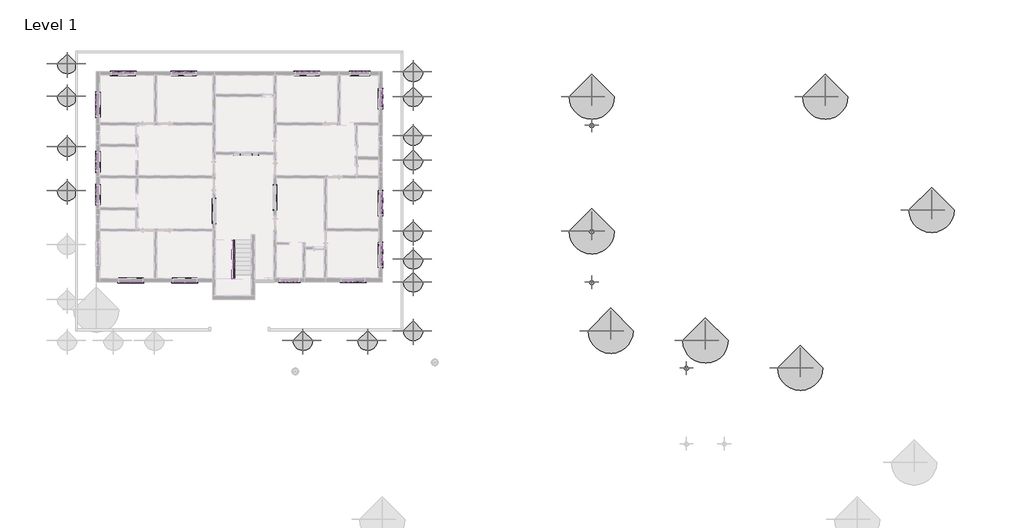
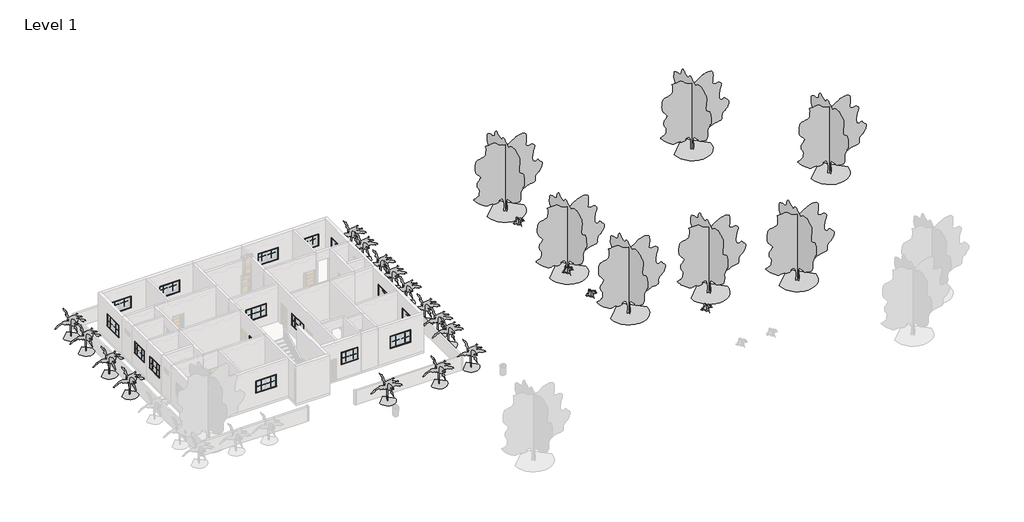
# One storey, part 5 of 5: 68 proxies, 26 geographic elements, 3 members.
"""IFC4 building model written with IfcOpenShell, lengths in millimetres."""

from ifc_helpers import new_model, si_unit, frame, origin, place, context, project, spatial, polyline, outline, extrude, transform, mapped, element, save
from components import m_muntin_pattern_2x2_m_muntin_pattern_2x2_9352d081, m_muntin_pattern_2x2_m_muntin_pattern_2x2_5c2cbe28, m_muntin_pattern_2x2_m_muntin_pattern_2x2_2357e71d, m_muntin_pattern_2x2_m_muntin_pattern_2x2_302d8f29, m_trim_window_exterior_flat_with_sill_e3533f3c, m_trim_window_exterior_flat_with_sill_6ae8fed8, m_trim_window_interior_flat_picture_frame_7d8195fd, m_trim_window_interior_flat_picture_frame_fffd0b6f, m_rpc_plant_tropical_agave_0_45_meters_eb57889b, m_rpc_tree_tropical_australian_tree_fern_1_8_meters_0203a3dd, rpc_tree_deciduous_american_beech_20_b3c041c8

model = new_model("IFC4")

# Units and contexts
model_context = context("Model", 3, world=origin())
ifc_project = project(units=[si_unit("LENGTHUNIT", "METRE", prefix="MILLI")], contexts=[model_context])

# Site, building, storey
site = spatial("IfcSite", under=ifc_project)
building = spatial("IfcBuilding", under=site)
storey = spatial("IfcBuildingStorey", under=building, Name="Level 1", Elevation=0.0)

# Proxies
placement = place(None, origin())
m_muntin_pattern_2x2_m_muntin_pattern_2x2_shape = m_muntin_pattern_2x2_m_muntin_pattern_2x2_9352d081(model_context)
element("IfcBuildingElementProxy", 1, Name="M_Muntin Pattern_2x2 : M_Muntin Pattern_2x2", ObjectType="M_Muntin Pattern_2x2 : M_Muntin Pattern_2x2", at=placement, inside=storey, context=model_context, shape_type="MappedRepresentation", body=[
    mapped(m_muntin_pattern_2x2_m_muntin_pattern_2x2_shape, transform((-23669.5972893, 23321.4672903, 1289.0070312), x_axis=(1.0, 0.0, 0.0), y_axis=(0.0, 1.0, 0.0), z_axis=(0.0, 0.0, 1.0))),
])
element("IfcBuildingElementProxy", 2, Name="M_Muntin Pattern_2x2 : M_Muntin Pattern_2x2", ObjectType="M_Muntin Pattern_2x2 : M_Muntin Pattern_2x2", at=placement, inside=storey, context=model_context, shape_type="MappedRepresentation", body=[
    mapped(m_muntin_pattern_2x2_m_muntin_pattern_2x2_shape, transform((-24995.1597893, 20843.3797903, 1289.0070312), x_axis=(0.0, 1.0, 0.0), y_axis=(-1.0, 0.0, 0.0), z_axis=(0.0, 0.0, 1.0))),
])
element("IfcBuildingElementProxy", 3, Name="M_Muntin Pattern_2x2 : M_Muntin Pattern_2x2", ObjectType="M_Muntin Pattern_2x2 : M_Muntin Pattern_2x2", at=placement, inside=storey, context=model_context, shape_type="MappedRepresentation", body=[
    mapped(m_muntin_pattern_2x2_m_muntin_pattern_2x2_shape, transform((-22415.4722893, 9802.3172903, 1289.0070312), x_axis=(-1.0, 0.0, 0.0), y_axis=(0.0, -1.0, 0.0), z_axis=(0.0, 0.0, 1.0))),
])
element("IfcBuildingElementProxy", 4, Name="M_Muntin Pattern_2x2 : M_Muntin Pattern_2x2", ObjectType="M_Muntin Pattern_2x2 : M_Muntin Pattern_2x2", at=placement, inside=storey, context=model_context, shape_type="MappedRepresentation", body=[
    mapped(m_muntin_pattern_2x2_m_muntin_pattern_2x2_shape, transform((-18935.6722893, 9802.3172903, 1289.0070312), x_axis=(-1.0, 0.0, 0.0), y_axis=(0.0, -1.0, 0.0), z_axis=(0.0, 0.0, 1.0))),
])
element("IfcBuildingElementProxy", 5, Name="M_Muntin Pattern_2x2 : M_Muntin Pattern_2x2", ObjectType="M_Muntin Pattern_2x2 : M_Muntin Pattern_2x2", at=placement, inside=storey, context=model_context, shape_type="MappedRepresentation", body=[
    mapped(m_muntin_pattern_2x2_m_muntin_pattern_2x2_shape, transform((-8121.6222893, 9827.7172903, 1289.0070312), x_axis=(-1.0, 0.0, 0.0), y_axis=(0.0, -1.0, 0.0), z_axis=(0.0, 0.0, 1.0))),
])
element("IfcBuildingElementProxy", 6, Name="M_Muntin Pattern_2x2 : M_Muntin Pattern_2x2", ObjectType="M_Muntin Pattern_2x2 : M_Muntin Pattern_2x2", at=placement, inside=storey, context=model_context, shape_type="MappedRepresentation", body=[
    mapped(m_muntin_pattern_2x2_m_muntin_pattern_2x2_shape, transform((-6624.6097893, 11931.1547903, 1289.0070312), x_axis=(0.0, -1.0, 0.0), y_axis=(1.0, 0.0, 0.0), z_axis=(0.0, 0.0, 1.0))),
])
element("IfcBuildingElementProxy", 7, Name="M_Muntin Pattern_2x2 : M_Muntin Pattern_2x2", ObjectType="M_Muntin Pattern_2x2 : M_Muntin Pattern_2x2", at=placement, inside=storey, context=model_context, shape_type="MappedRepresentation", body=[
    mapped(m_muntin_pattern_2x2_m_muntin_pattern_2x2_shape, transform((-6624.6097893, 15252.2047903, 1289.0070312), x_axis=(0.0, -1.0, 0.0), y_axis=(1.0, 0.0, 0.0), z_axis=(0.0, 0.0, 1.0))),
])
element("IfcBuildingElementProxy", 8, Name="M_Muntin Pattern_2x2 : M_Muntin Pattern_2x2", ObjectType="M_Muntin Pattern_2x2 : M_Muntin Pattern_2x2", at=placement, inside=storey, context=model_context, shape_type="MappedRepresentation", body=[
    mapped(m_muntin_pattern_2x2_m_muntin_pattern_2x2_shape, transform((-11845.8972893, 23321.4672903, 1289.0070312), x_axis=(1.0, 0.0, 0.0), y_axis=(0.0, 1.0, 0.0), z_axis=(0.0, 0.0, 1.0))),
])
element("IfcBuildingElementProxy", 9, Name="M_Muntin Pattern_2x2 : M_Muntin Pattern_2x2", ObjectType="M_Muntin Pattern_2x2 : M_Muntin Pattern_2x2", at=placement, inside=storey, context=model_context, shape_type="MappedRepresentation", body=[
    mapped(m_muntin_pattern_2x2_m_muntin_pattern_2x2_shape, transform((-19770.6972893, 23321.4672903, 1289.0070312), x_axis=(1.0, 0.0, 0.0), y_axis=(0.0, 1.0, 0.0), z_axis=(0.0, 0.0, 1.0))),
])
element("IfcBuildingElementProxy", 10, Name="M_Muntin Pattern_2x2 : M_Muntin Pattern_2x2", ObjectType="M_Muntin Pattern_2x2 : M_Muntin Pattern_2x2", at=placement, inside=storey, context=model_context, shape_type="MappedRepresentation", body=[
    mapped(m_muntin_pattern_2x2_m_muntin_pattern_2x2_shape, transform((-14998.6722893, 18006.5172903, 969.85), x_axis=(-1.0, 0.0, 0.0), y_axis=(0.0, -1.0, 0.0), z_axis=(0.0, 0.0, 1.0))),
])
element("IfcBuildingElementProxy", 11, Name="M_Muntin Pattern_2x2 : M_Muntin Pattern_2x2", ObjectType="M_Muntin Pattern_2x2 : M_Muntin Pattern_2x2", at=placement, inside=storey, context=model_context, shape_type="MappedRepresentation", body=[
    mapped(m_muntin_pattern_2x2_m_muntin_pattern_2x2_shape, transform((-17368.8097893, 14744.2047903, 969.85), x_axis=(0.0, -1.0, 0.0), y_axis=(1.0, 0.0, 0.0), z_axis=(0.0, 0.0, 1.0))),
])
element("IfcBuildingElementProxy", 12, Name="M_Muntin Pattern_2x2 : M_Muntin Pattern_2x2", ObjectType="M_Muntin Pattern_2x2 : M_Muntin Pattern_2x2", at=placement, inside=storey, context=model_context, shape_type="MappedRepresentation", body=[
    mapped(m_muntin_pattern_2x2_m_muntin_pattern_2x2_shape, transform((-13590.5597893, 14874.3797903, 969.85), x_axis=(0.0, 1.0, 0.0), y_axis=(-1.0, 0.0, 0.0), z_axis=(0.0, 0.0, 1.0))),
])
m_muntin_pattern_2x2_m_muntin_pattern_2x2_2_shape = m_muntin_pattern_2x2_m_muntin_pattern_2x2_5c2cbe28(model_context)
element("IfcBuildingElementProxy", 13, Name="M_Muntin Pattern_2x2 : M_Muntin Pattern_2x2", ObjectType="M_Muntin Pattern_2x2 : M_Muntin Pattern_2x2", at=placement, inside=storey, context=model_context, shape_type="MappedRepresentation", body=[
    mapped(m_muntin_pattern_2x2_m_muntin_pattern_2x2_2_shape, transform((-22910.7722893, 23321.4672903, 1289.0070313), x_axis=(-1.0, 0.0, 0.0), y_axis=(0.0, -1.0, 0.0), z_axis=(0.0, 0.0, 1.0))),
])
element("IfcBuildingElementProxy", 14, Name="M_Muntin Pattern_2x2 : M_Muntin Pattern_2x2", ObjectType="M_Muntin Pattern_2x2 : M_Muntin Pattern_2x2", at=placement, inside=storey, context=model_context, shape_type="MappedRepresentation", body=[
    mapped(m_muntin_pattern_2x2_m_muntin_pattern_2x2_2_shape, transform((-24995.1597893, 21602.2047903, 1289.0070313), x_axis=(0.0, -1.0, 0.0), y_axis=(1.0, 0.0, 0.0), z_axis=(0.0, 0.0, 1.0))),
])
element("IfcBuildingElementProxy", 15, Name="M_Muntin Pattern_2x2 : M_Muntin Pattern_2x2", ObjectType="M_Muntin Pattern_2x2 : M_Muntin Pattern_2x2", at=placement, inside=storey, context=model_context, shape_type="MappedRepresentation", body=[
    mapped(m_muntin_pattern_2x2_m_muntin_pattern_2x2_2_shape, transform((-23174.2972893, 9802.3172903, 1289.0070313), x_axis=(1.0, 0.0, 0.0), y_axis=(0.0, 1.0, 0.0), z_axis=(0.0, 0.0, 1.0))),
])
element("IfcBuildingElementProxy", 16, Name="M_Muntin Pattern_2x2 : M_Muntin Pattern_2x2", ObjectType="M_Muntin Pattern_2x2 : M_Muntin Pattern_2x2", at=placement, inside=storey, context=model_context, shape_type="MappedRepresentation", body=[
    mapped(m_muntin_pattern_2x2_m_muntin_pattern_2x2_2_shape, transform((-19694.4972893, 9802.3172903, 1289.0070313), x_axis=(1.0, 0.0, 0.0), y_axis=(0.0, 1.0, 0.0), z_axis=(0.0, 0.0, 1.0))),
])
element("IfcBuildingElementProxy", 17, Name="M_Muntin Pattern_2x2 : M_Muntin Pattern_2x2", ObjectType="M_Muntin Pattern_2x2 : M_Muntin Pattern_2x2", at=placement, inside=storey, context=model_context, shape_type="MappedRepresentation", body=[
    mapped(m_muntin_pattern_2x2_m_muntin_pattern_2x2_2_shape, transform((-8880.4472893, 9827.7172903, 1289.0070313), x_axis=(1.0, 0.0, 0.0), y_axis=(0.0, 1.0, 0.0), z_axis=(0.0, 0.0, 1.0))),
])
element("IfcBuildingElementProxy", 18, Name="M_Muntin Pattern_2x2 : M_Muntin Pattern_2x2", ObjectType="M_Muntin Pattern_2x2 : M_Muntin Pattern_2x2", at=placement, inside=storey, context=model_context, shape_type="MappedRepresentation", body=[
    mapped(m_muntin_pattern_2x2_m_muntin_pattern_2x2_2_shape, transform((-6624.6097893, 11172.3297903, 1289.0070313), x_axis=(0.0, 1.0, 0.0), y_axis=(-1.0, 0.0, 0.0), z_axis=(0.0, 0.0, 1.0))),
])
element("IfcBuildingElementProxy", 19, Name="M_Muntin Pattern_2x2 : M_Muntin Pattern_2x2", ObjectType="M_Muntin Pattern_2x2 : M_Muntin Pattern_2x2", at=placement, inside=storey, context=model_context, shape_type="MappedRepresentation", body=[
    mapped(m_muntin_pattern_2x2_m_muntin_pattern_2x2_2_shape, transform((-6624.6097893, 14493.3797903, 1289.0070313), x_axis=(0.0, 1.0, 0.0), y_axis=(-1.0, 0.0, 0.0), z_axis=(0.0, 0.0, 1.0))),
])
element("IfcBuildingElementProxy", 20, Name="M_Muntin Pattern_2x2 : M_Muntin Pattern_2x2", ObjectType="M_Muntin Pattern_2x2 : M_Muntin Pattern_2x2", at=placement, inside=storey, context=model_context, shape_type="MappedRepresentation", body=[
    mapped(m_muntin_pattern_2x2_m_muntin_pattern_2x2_2_shape, transform((-11087.0722893, 23321.4672903, 1289.0070313), x_axis=(-1.0, 0.0, 0.0), y_axis=(0.0, -1.0, 0.0), z_axis=(0.0, 0.0, 1.0))),
])
element("IfcBuildingElementProxy", 21, Name="M_Muntin Pattern_2x2 : M_Muntin Pattern_2x2", ObjectType="M_Muntin Pattern_2x2 : M_Muntin Pattern_2x2", at=placement, inside=storey, context=model_context, shape_type="MappedRepresentation", body=[
    mapped(m_muntin_pattern_2x2_m_muntin_pattern_2x2_2_shape, transform((-19011.8722893, 23321.4672903, 1289.0070313), x_axis=(-1.0, 0.0, 0.0), y_axis=(0.0, -1.0, 0.0), z_axis=(0.0, 0.0, 1.0))),
])
element("IfcBuildingElementProxy", 22, Name="M_Muntin Pattern_2x2 : M_Muntin Pattern_2x2", ObjectType="M_Muntin Pattern_2x2 : M_Muntin Pattern_2x2", at=placement, inside=storey, context=model_context, shape_type="MappedRepresentation", body=[
    mapped(m_muntin_pattern_2x2_m_muntin_pattern_2x2_2_shape, transform((-15757.4972893, 18006.5172903, 969.85), x_axis=(1.0, 0.0, 0.0), y_axis=(0.0, 1.0, 0.0), z_axis=(0.0, 0.0, 1.0))),
])
element("IfcBuildingElementProxy", 23, Name="M_Muntin Pattern_2x2 : M_Muntin Pattern_2x2", ObjectType="M_Muntin Pattern_2x2 : M_Muntin Pattern_2x2", at=placement, inside=storey, context=model_context, shape_type="MappedRepresentation", body=[
    mapped(m_muntin_pattern_2x2_m_muntin_pattern_2x2_2_shape, transform((-17368.8097893, 13985.3797903, 969.85), x_axis=(0.0, 1.0, 0.0), y_axis=(-1.0, 0.0, 0.0), z_axis=(0.0, 0.0, 1.0))),
])
element("IfcBuildingElementProxy", 24, Name="M_Muntin Pattern_2x2 : M_Muntin Pattern_2x2", ObjectType="M_Muntin Pattern_2x2 : M_Muntin Pattern_2x2", at=placement, inside=storey, context=model_context, shape_type="MappedRepresentation", body=[
    mapped(m_muntin_pattern_2x2_m_muntin_pattern_2x2_2_shape, transform((-13590.5597893, 15633.2047903, 969.85), x_axis=(0.0, -1.0, 0.0), y_axis=(1.0, 0.0, 0.0), z_axis=(0.0, 0.0, 1.0))),
])
m_muntin_pattern_2x2_m_muntin_pattern_2x2_3_shape = m_muntin_pattern_2x2_m_muntin_pattern_2x2_2357e71d(model_context)
element("IfcBuildingElementProxy", 25, Name="M_Muntin Pattern_2x2 : M_Muntin Pattern_2x2", ObjectType="M_Muntin Pattern_2x2 : M_Muntin Pattern_2x2", at=placement, inside=storey, context=model_context, shape_type="MappedRepresentation", body=[
    mapped(m_muntin_pattern_2x2_m_muntin_pattern_2x2_3_shape, transform((-24995.1597893, 17236.5797903, 1289.05), x_axis=(0.0, 1.0, 0.0), y_axis=(-1.0, 0.0, 0.0), z_axis=(0.0, 0.0, 1.0))),
])
element("IfcBuildingElementProxy", 26, Name="M_Muntin Pattern_2x2 : M_Muntin Pattern_2x2", ObjectType="M_Muntin Pattern_2x2 : M_Muntin Pattern_2x2", at=placement, inside=storey, context=model_context, shape_type="MappedRepresentation", body=[
    mapped(m_muntin_pattern_2x2_m_muntin_pattern_2x2_3_shape, transform((-24995.1597893, 15128.3797903, 1289.05), x_axis=(0.0, 1.0, 0.0), y_axis=(-1.0, 0.0, 0.0), z_axis=(0.0, 0.0, 1.0))),
])
element("IfcBuildingElementProxy", 27, Name="M_Muntin Pattern_2x2 : M_Muntin Pattern_2x2", ObjectType="M_Muntin Pattern_2x2 : M_Muntin Pattern_2x2", at=placement, inside=storey, context=model_context, shape_type="MappedRepresentation", body=[
    mapped(m_muntin_pattern_2x2_m_muntin_pattern_2x2_3_shape, transform((-12280.8722893, 9827.7172903, 1289.05), x_axis=(-1.0, 0.0, 0.0), y_axis=(0.0, -1.0, 0.0), z_axis=(0.0, 0.0, 1.0))),
])
element("IfcBuildingElementProxy", 28, Name="M_Muntin Pattern_2x2 : M_Muntin Pattern_2x2", ObjectType="M_Muntin Pattern_2x2 : M_Muntin Pattern_2x2", at=placement, inside=storey, context=model_context, shape_type="MappedRepresentation", body=[
    mapped(m_muntin_pattern_2x2_m_muntin_pattern_2x2_3_shape, transform((-6624.6097893, 21900.6547903, 1289.05), x_axis=(0.0, -1.0, 0.0), y_axis=(1.0, 0.0, 0.0), z_axis=(0.0, 0.0, 1.0))),
])
element("IfcBuildingElementProxy", 29, Name="M_Muntin Pattern_2x2 : M_Muntin Pattern_2x2", ObjectType="M_Muntin Pattern_2x2 : M_Muntin Pattern_2x2", at=placement, inside=storey, context=model_context, shape_type="MappedRepresentation", body=[
    mapped(m_muntin_pattern_2x2_m_muntin_pattern_2x2_3_shape, transform((-8372.4472893, 23321.4672903, 1289.05), x_axis=(1.0, 0.0, 0.0), y_axis=(0.0, 1.0, 0.0), z_axis=(0.0, 0.0, 1.0))),
])
m_muntin_pattern_2x2_m_muntin_pattern_2x2_4_shape = m_muntin_pattern_2x2_m_muntin_pattern_2x2_302d8f29(model_context)
element("IfcBuildingElementProxy", 30, Name="M_Muntin Pattern_2x2 : M_Muntin Pattern_2x2", ObjectType="M_Muntin Pattern_2x2 : M_Muntin Pattern_2x2", at=placement, inside=storey, context=model_context, shape_type="MappedRepresentation", body=[
    mapped(m_muntin_pattern_2x2_m_muntin_pattern_2x2_4_shape, transform((-24995.1597893, 17843.0047903, 1289.05), x_axis=(0.0, -1.0, 0.0), y_axis=(1.0, 0.0, 0.0), z_axis=(0.0, 0.0, 1.0))),
])
element("IfcBuildingElementProxy", 31, Name="M_Muntin Pattern_2x2 : M_Muntin Pattern_2x2", ObjectType="M_Muntin Pattern_2x2 : M_Muntin Pattern_2x2", at=placement, inside=storey, context=model_context, shape_type="MappedRepresentation", body=[
    mapped(m_muntin_pattern_2x2_m_muntin_pattern_2x2_4_shape, transform((-24995.1597893, 15734.8047903, 1289.05), x_axis=(0.0, -1.0, 0.0), y_axis=(1.0, 0.0, 0.0), z_axis=(0.0, 0.0, 1.0))),
])
element("IfcBuildingElementProxy", 32, Name="M_Muntin Pattern_2x2 : M_Muntin Pattern_2x2", ObjectType="M_Muntin Pattern_2x2 : M_Muntin Pattern_2x2", at=placement, inside=storey, context=model_context, shape_type="MappedRepresentation", body=[
    mapped(m_muntin_pattern_2x2_m_muntin_pattern_2x2_4_shape, transform((-12887.2972893, 9827.7172903, 1289.05), x_axis=(1.0, 0.0, 0.0), y_axis=(0.0, 1.0, 0.0), z_axis=(0.0, 0.0, 1.0))),
])
element("IfcBuildingElementProxy", 33, Name="M_Muntin Pattern_2x2 : M_Muntin Pattern_2x2", ObjectType="M_Muntin Pattern_2x2 : M_Muntin Pattern_2x2", at=placement, inside=storey, context=model_context, shape_type="MappedRepresentation", body=[
    mapped(m_muntin_pattern_2x2_m_muntin_pattern_2x2_4_shape, transform((-6624.6097893, 21294.2297903, 1289.05), x_axis=(0.0, 1.0, 0.0), y_axis=(-1.0, 0.0, 0.0), z_axis=(0.0, 0.0, 1.0))),
])
element("IfcBuildingElementProxy", 34, Name="M_Muntin Pattern_2x2 : M_Muntin Pattern_2x2", ObjectType="M_Muntin Pattern_2x2 : M_Muntin Pattern_2x2", at=placement, inside=storey, context=model_context, shape_type="MappedRepresentation", body=[
    mapped(m_muntin_pattern_2x2_m_muntin_pattern_2x2_4_shape, transform((-7766.0222893, 23321.4672903, 1289.05), x_axis=(-1.0, 0.0, 0.0), y_axis=(0.0, -1.0, 0.0), z_axis=(0.0, 0.0, 1.0))),
])
m_trim_window_exterior_flat_with_sill_shape = m_trim_window_exterior_flat_with_sill_e3533f3c(model_context)
element("IfcBuildingElementProxy", 35, Name="M_Trim-Window-Exterior-Flat : with Sill", ObjectType="M_Trim-Window-Exterior-Flat : with Sill", at=placement, inside=storey, context=model_context, shape_type="MappedRepresentation", body=[
    mapped(m_trim_window_exterior_flat_with_sill_shape, transform((-23290.1847893, 23330.9922903, 2133.5570313), x_axis=(-1.0, 0.0, 0.0), y_axis=(0.0, 0.0, 1.0), z_axis=(0.0, 1.0, 0.0))),
])
element("IfcBuildingElementProxy", 36, Name="M_Trim-Window-Exterior-Flat : with Sill", ObjectType="M_Trim-Window-Exterior-Flat : with Sill", at=placement, inside=storey, context=model_context, shape_type="MappedRepresentation", body=[
    mapped(m_trim_window_exterior_flat_with_sill_shape, transform((-25004.6847893, 21222.7922903, 2133.5570313), x_axis=(0.0, -1.0, 0.0), y_axis=(0.0, 0.0, 1.0), z_axis=(-1.0, 0.0, 0.0))),
])
element("IfcBuildingElementProxy", 37, Name="M_Trim-Window-Exterior-Flat : with Sill", ObjectType="M_Trim-Window-Exterior-Flat : with Sill", at=placement, inside=storey, context=model_context, shape_type="MappedRepresentation", body=[
    mapped(m_trim_window_exterior_flat_with_sill_shape, transform((-22794.8847893, 9792.7922903, 2133.5570313), x_axis=(1.0, 0.0, 0.0), y_axis=(0.0, 0.0, 1.0), z_axis=(0.0, -1.0, 0.0))),
])
element("IfcBuildingElementProxy", 38, Name="M_Trim-Window-Exterior-Flat : with Sill", ObjectType="M_Trim-Window-Exterior-Flat : with Sill", at=placement, inside=storey, context=model_context, shape_type="MappedRepresentation", body=[
    mapped(m_trim_window_exterior_flat_with_sill_shape, transform((-19315.0847893, 9792.7922903, 2133.5570313), x_axis=(1.0, 0.0, 0.0), y_axis=(0.0, 0.0, 1.0), z_axis=(0.0, -1.0, 0.0))),
])
element("IfcBuildingElementProxy", 39, Name="M_Trim-Window-Exterior-Flat : with Sill", ObjectType="M_Trim-Window-Exterior-Flat : with Sill", at=placement, inside=storey, context=model_context, shape_type="MappedRepresentation", body=[
    mapped(m_trim_window_exterior_flat_with_sill_shape, transform((-8501.0347893, 9818.1922903, 2133.5570313), x_axis=(1.0, 0.0, 0.0), y_axis=(0.0, 0.0, 1.0), z_axis=(0.0, -1.0, 0.0))),
])
element("IfcBuildingElementProxy", 40, Name="M_Trim-Window-Exterior-Flat : with Sill", ObjectType="M_Trim-Window-Exterior-Flat : with Sill", at=placement, inside=storey, context=model_context, shape_type="MappedRepresentation", body=[
    mapped(m_trim_window_exterior_flat_with_sill_shape, transform((-6615.0847893, 11551.7422903, 2133.5570313), x_axis=(0.0, 1.0, 0.0), y_axis=(0.0, 0.0, 1.0), z_axis=(1.0, 0.0, 0.0))),
])
element("IfcBuildingElementProxy", 41, Name="M_Trim-Window-Exterior-Flat : with Sill", ObjectType="M_Trim-Window-Exterior-Flat : with Sill", at=placement, inside=storey, context=model_context, shape_type="MappedRepresentation", body=[
    mapped(m_trim_window_exterior_flat_with_sill_shape, transform((-6615.0847893, 14872.7922903, 2133.5570313), x_axis=(0.0, 1.0, 0.0), y_axis=(0.0, 0.0, 1.0), z_axis=(1.0, 0.0, 0.0))),
])
element("IfcBuildingElementProxy", 42, Name="M_Trim-Window-Exterior-Flat : with Sill", ObjectType="M_Trim-Window-Exterior-Flat : with Sill", at=placement, inside=storey, context=model_context, shape_type="MappedRepresentation", body=[
    mapped(m_trim_window_exterior_flat_with_sill_shape, transform((-11466.4847893, 23330.9922903, 2133.5570313), x_axis=(-1.0, 0.0, 0.0), y_axis=(0.0, 0.0, 1.0), z_axis=(0.0, 1.0, 0.0))),
])
element("IfcBuildingElementProxy", 43, Name="M_Trim-Window-Exterior-Flat : with Sill", ObjectType="M_Trim-Window-Exterior-Flat : with Sill", at=placement, inside=storey, context=model_context, shape_type="MappedRepresentation", body=[
    mapped(m_trim_window_exterior_flat_with_sill_shape, transform((-19391.2847893, 23330.9922903, 2133.5570313), x_axis=(-1.0, 0.0, 0.0), y_axis=(0.0, 0.0, 1.0), z_axis=(0.0, 1.0, 0.0))),
])
element("IfcBuildingElementProxy", 44, Name="M_Trim-Window-Exterior-Flat : with Sill", ObjectType="M_Trim-Window-Exterior-Flat : with Sill", at=placement, inside=storey, context=model_context, shape_type="MappedRepresentation", body=[
    mapped(m_trim_window_exterior_flat_with_sill_shape, transform((-15378.0847893, 17996.9922903, 1814.4), x_axis=(1.0, 0.0, 0.0), y_axis=(0.0, 0.0, 1.0), z_axis=(0.0, -1.0, 0.0))),
])
element("IfcBuildingElementProxy", 45, Name="M_Trim-Window-Exterior-Flat : with Sill", ObjectType="M_Trim-Window-Exterior-Flat : with Sill", at=placement, inside=storey, context=model_context, shape_type="MappedRepresentation", body=[
    mapped(m_trim_window_exterior_flat_with_sill_shape, transform((-17359.2847893, 14364.7922903, 1814.4), x_axis=(0.0, 1.0, 0.0), y_axis=(0.0, 0.0, 1.0), z_axis=(1.0, 0.0, 0.0))),
])
element("IfcBuildingElementProxy", 46, Name="M_Trim-Window-Exterior-Flat : with Sill", ObjectType="M_Trim-Window-Exterior-Flat : with Sill", at=placement, inside=storey, context=model_context, shape_type="MappedRepresentation", body=[
    mapped(m_trim_window_exterior_flat_with_sill_shape, transform((-13600.0847893, 15253.7922903, 1814.4), x_axis=(0.0, -1.0, 0.0), y_axis=(0.0, 0.0, 1.0), z_axis=(-1.0, 0.0, 0.0))),
])
m_trim_window_exterior_flat_with_sill_2_shape = m_trim_window_exterior_flat_with_sill_6ae8fed8(model_context)
element("IfcBuildingElementProxy", 47, Name="M_Trim-Window-Exterior-Flat : with Sill", ObjectType="M_Trim-Window-Exterior-Flat : with Sill", at=placement, inside=storey, context=model_context, shape_type="MappedRepresentation", body=[
    mapped(m_trim_window_exterior_flat_with_sill_2_shape, transform((-25004.6847893, 17539.7922903, 2133.6), x_axis=(0.0, -1.0, 0.0), y_axis=(0.0, 0.0, 1.0), z_axis=(-1.0, 0.0, 0.0))),
])
element("IfcBuildingElementProxy", 48, Name="M_Trim-Window-Exterior-Flat : with Sill", ObjectType="M_Trim-Window-Exterior-Flat : with Sill", at=placement, inside=storey, context=model_context, shape_type="MappedRepresentation", body=[
    mapped(m_trim_window_exterior_flat_with_sill_2_shape, transform((-25004.6847893, 15431.5922903, 2133.6), x_axis=(0.0, -1.0, 0.0), y_axis=(0.0, 0.0, 1.0), z_axis=(-1.0, 0.0, 0.0))),
])
element("IfcBuildingElementProxy", 49, Name="M_Trim-Window-Exterior-Flat : with Sill", ObjectType="M_Trim-Window-Exterior-Flat : with Sill", at=placement, inside=storey, context=model_context, shape_type="MappedRepresentation", body=[
    mapped(m_trim_window_exterior_flat_with_sill_2_shape, transform((-12584.0847893, 9818.1922903, 2133.6), x_axis=(1.0, 0.0, 0.0), y_axis=(0.0, 0.0, 1.0), z_axis=(0.0, -1.0, 0.0))),
])
element("IfcBuildingElementProxy", 50, Name="M_Trim-Window-Exterior-Flat : with Sill", ObjectType="M_Trim-Window-Exterior-Flat : with Sill", at=placement, inside=storey, context=model_context, shape_type="MappedRepresentation", body=[
    mapped(m_trim_window_exterior_flat_with_sill_2_shape, transform((-6615.0847893, 21597.4422903, 2133.6), x_axis=(0.0, 1.0, 0.0), y_axis=(0.0, 0.0, 1.0), z_axis=(1.0, 0.0, 0.0))),
])
element("IfcBuildingElementProxy", 51, Name="M_Trim-Window-Exterior-Flat : with Sill", ObjectType="M_Trim-Window-Exterior-Flat : with Sill", at=placement, inside=storey, context=model_context, shape_type="MappedRepresentation", body=[
    mapped(m_trim_window_exterior_flat_with_sill_2_shape, transform((-8069.2347893, 23330.9922903, 2133.6), x_axis=(-1.0, 0.0, 0.0), y_axis=(0.0, 0.0, 1.0), z_axis=(0.0, 1.0, 0.0))),
])
m_trim_window_interior_flat_picture_frame_shape = m_trim_window_interior_flat_picture_frame_7d8195fd(model_context)
element("IfcBuildingElementProxy", 52, Name="M_Trim-Window-Interior-Flat : Picture Frame", ObjectType="M_Trim-Window-Interior-Flat : Picture Frame", at=placement, inside=storey, context=model_context, shape_type="MappedRepresentation", body=[
    mapped(m_trim_window_interior_flat_picture_frame_shape, transform((-23290.1847893, 23102.3922903, 2133.5570313), x_axis=(1.0, 0.0, 0.0), y_axis=(0.0, 0.0, 1.0), z_axis=(0.0, -1.0, 0.0))),
])
element("IfcBuildingElementProxy", 53, Name="M_Trim-Window-Interior-Flat : Picture Frame", ObjectType="M_Trim-Window-Interior-Flat : Picture Frame", at=placement, inside=storey, context=model_context, shape_type="MappedRepresentation", body=[
    mapped(m_trim_window_interior_flat_picture_frame_shape, transform((-24776.0847893, 21222.7922903, 2133.5570313), x_axis=(0.0, 1.0, 0.0), y_axis=(0.0, 0.0, 1.0), z_axis=(1.0, 0.0, 0.0))),
])
element("IfcBuildingElementProxy", 54, Name="M_Trim-Window-Interior-Flat : Picture Frame", ObjectType="M_Trim-Window-Interior-Flat : Picture Frame", at=placement, inside=storey, context=model_context, shape_type="MappedRepresentation", body=[
    mapped(m_trim_window_interior_flat_picture_frame_shape, transform((-22794.8847893, 10021.3922903, 2133.5570313), x_axis=(-1.0, 0.0, 0.0), y_axis=(0.0, 0.0, 1.0), z_axis=(0.0, 1.0, 0.0))),
])
element("IfcBuildingElementProxy", 55, Name="M_Trim-Window-Interior-Flat : Picture Frame", ObjectType="M_Trim-Window-Interior-Flat : Picture Frame", at=placement, inside=storey, context=model_context, shape_type="MappedRepresentation", body=[
    mapped(m_trim_window_interior_flat_picture_frame_shape, transform((-19315.0847893, 10021.3922903, 2133.5570313), x_axis=(-1.0, 0.0, 0.0), y_axis=(0.0, 0.0, 1.0), z_axis=(0.0, 1.0, 0.0))),
])
element("IfcBuildingElementProxy", 56, Name="M_Trim-Window-Interior-Flat : Picture Frame", ObjectType="M_Trim-Window-Interior-Flat : Picture Frame", at=placement, inside=storey, context=model_context, shape_type="MappedRepresentation", body=[
    mapped(m_trim_window_interior_flat_picture_frame_shape, transform((-8501.0347893, 10046.7922903, 2133.5570313), x_axis=(-1.0, 0.0, 0.0), y_axis=(0.0, 0.0, 1.0), z_axis=(0.0, 1.0, 0.0))),
])
element("IfcBuildingElementProxy", 57, Name="M_Trim-Window-Interior-Flat : Picture Frame", ObjectType="M_Trim-Window-Interior-Flat : Picture Frame", at=placement, inside=storey, context=model_context, shape_type="MappedRepresentation", body=[
    mapped(m_trim_window_interior_flat_picture_frame_shape, transform((-6843.6847893, 11551.7422903, 2133.5570313), x_axis=(0.0, -1.0, 0.0), y_axis=(0.0, 0.0, 1.0), z_axis=(-1.0, 0.0, 0.0))),
])
element("IfcBuildingElementProxy", 58, Name="M_Trim-Window-Interior-Flat : Picture Frame", ObjectType="M_Trim-Window-Interior-Flat : Picture Frame", at=placement, inside=storey, context=model_context, shape_type="MappedRepresentation", body=[
    mapped(m_trim_window_interior_flat_picture_frame_shape, transform((-6843.6847893, 14872.7922903, 2133.5570313), x_axis=(0.0, -1.0, 0.0), y_axis=(0.0, 0.0, 1.0), z_axis=(-1.0, 0.0, 0.0))),
])
element("IfcBuildingElementProxy", 59, Name="M_Trim-Window-Interior-Flat : Picture Frame", ObjectType="M_Trim-Window-Interior-Flat : Picture Frame", at=placement, inside=storey, context=model_context, shape_type="MappedRepresentation", body=[
    mapped(m_trim_window_interior_flat_picture_frame_shape, transform((-11466.4847893, 23102.3922903, 2133.5570313), x_axis=(1.0, 0.0, 0.0), y_axis=(0.0, 0.0, 1.0), z_axis=(0.0, -1.0, 0.0))),
])
element("IfcBuildingElementProxy", 60, Name="M_Trim-Window-Interior-Flat : Picture Frame", ObjectType="M_Trim-Window-Interior-Flat : Picture Frame", at=placement, inside=storey, context=model_context, shape_type="MappedRepresentation", body=[
    mapped(m_trim_window_interior_flat_picture_frame_shape, transform((-19391.2847893, 23102.3922903, 2133.5570313), x_axis=(1.0, 0.0, 0.0), y_axis=(0.0, 0.0, 1.0), z_axis=(0.0, -1.0, 0.0))),
])
element("IfcBuildingElementProxy", 61, Name="M_Trim-Window-Interior-Flat : Picture Frame", ObjectType="M_Trim-Window-Interior-Flat : Picture Frame", at=placement, inside=storey, context=model_context, shape_type="MappedRepresentation", body=[
    mapped(m_trim_window_interior_flat_picture_frame_shape, transform((-15378.0847893, 18149.3922903, 1814.4), x_axis=(-1.0, 0.0, 0.0), y_axis=(0.0, 0.0, 1.0), z_axis=(0.0, 1.0, 0.0))),
])
element("IfcBuildingElementProxy", 62, Name="M_Trim-Window-Interior-Flat : Picture Frame", ObjectType="M_Trim-Window-Interior-Flat : Picture Frame", at=placement, inside=storey, context=model_context, shape_type="MappedRepresentation", body=[
    mapped(m_trim_window_interior_flat_picture_frame_shape, transform((-17511.6847893, 14364.7922903, 1814.4), x_axis=(0.0, -1.0, 0.0), y_axis=(0.0, 0.0, 1.0), z_axis=(-1.0, 0.0, 0.0))),
])
element("IfcBuildingElementProxy", 63, Name="M_Trim-Window-Interior-Flat : Picture Frame", ObjectType="M_Trim-Window-Interior-Flat : Picture Frame", at=placement, inside=storey, context=model_context, shape_type="MappedRepresentation", body=[
    mapped(m_trim_window_interior_flat_picture_frame_shape, transform((-13447.6847893, 15253.7922903, 1814.4), x_axis=(0.0, 1.0, 0.0), y_axis=(0.0, 0.0, 1.0), z_axis=(1.0, 0.0, 0.0))),
])
m_trim_window_interior_flat_picture_frame_2_shape = m_trim_window_interior_flat_picture_frame_fffd0b6f(model_context)
element("IfcBuildingElementProxy", 64, Name="M_Trim-Window-Interior-Flat : Picture Frame", ObjectType="M_Trim-Window-Interior-Flat : Picture Frame", at=placement, inside=storey, context=model_context, shape_type="MappedRepresentation", body=[
    mapped(m_trim_window_interior_flat_picture_frame_2_shape, transform((-24776.0847893, 17539.7922903, 2133.6), x_axis=(0.0, 1.0, 0.0), y_axis=(0.0, 0.0, 1.0), z_axis=(1.0, 0.0, 0.0))),
])
element("IfcBuildingElementProxy", 65, Name="M_Trim-Window-Interior-Flat : Picture Frame", ObjectType="M_Trim-Window-Interior-Flat : Picture Frame", at=placement, inside=storey, context=model_context, shape_type="MappedRepresentation", body=[
    mapped(m_trim_window_interior_flat_picture_frame_2_shape, transform((-24776.0847893, 15431.5922903, 2133.6), x_axis=(0.0, 1.0, 0.0), y_axis=(0.0, 0.0, 1.0), z_axis=(1.0, 0.0, 0.0))),
])
element("IfcBuildingElementProxy", 66, Name="M_Trim-Window-Interior-Flat : Picture Frame", ObjectType="M_Trim-Window-Interior-Flat : Picture Frame", at=placement, inside=storey, context=model_context, shape_type="MappedRepresentation", body=[
    mapped(m_trim_window_interior_flat_picture_frame_2_shape, transform((-12584.0847893, 10046.7922903, 2133.6), x_axis=(-1.0, 0.0, 0.0), y_axis=(0.0, 0.0, 1.0), z_axis=(0.0, 1.0, 0.0))),
])
element("IfcBuildingElementProxy", 67, Name="M_Trim-Window-Interior-Flat : Picture Frame", ObjectType="M_Trim-Window-Interior-Flat : Picture Frame", at=placement, inside=storey, context=model_context, shape_type="MappedRepresentation", body=[
    mapped(m_trim_window_interior_flat_picture_frame_2_shape, transform((-6843.6847893, 21597.4422903, 2133.6), x_axis=(0.0, -1.0, 0.0), y_axis=(0.0, 0.0, 1.0), z_axis=(-1.0, 0.0, 0.0))),
])
element("IfcBuildingElementProxy", 68, Name="M_Trim-Window-Interior-Flat : Picture Frame", ObjectType="M_Trim-Window-Interior-Flat : Picture Frame", at=placement, inside=storey, context=model_context, shape_type="MappedRepresentation", body=[
    mapped(m_trim_window_interior_flat_picture_frame_2_shape, transform((-8069.2347893, 23102.3922903, 2133.6), x_axis=(1.0, 0.0, 0.0), y_axis=(0.0, 0.0, 1.0), z_axis=(0.0, -1.0, 0.0))),
])

# Geographic elements
m_rpc_plant_tropical_agave_0_45_meters_shape = m_rpc_plant_tropical_agave_0_45_meters_eb57889b(model_context)
element("IfcGeographicElement", 69, ObjectType="M_RPC Plant - Tropical : Agave - 0.45 Meters", at=placement, inside=storey, context=model_context, shape_type="MappedRepresentation", body=[
    mapped(m_rpc_plant_tropical_agave_0_45_meters_shape, transform((6846.7185396, 19901.9922903, 0.0), x_axis=(1.0, 0.0, 0.0), y_axis=(0.0, 1.0, 0.0), z_axis=(0.0, 0.0, 1.0))),
])
element("IfcGeographicElement", 70, ObjectType="M_RPC Plant - Tropical : Agave - 0.45 Meters", at=placement, inside=storey, context=model_context, shape_type="MappedRepresentation", body=[
    mapped(m_rpc_plant_tropical_agave_0_45_meters_shape, transform((6846.7185396, 13069.3922903, 0.0), x_axis=(1.0, 0.0, 0.0), y_axis=(0.0, 1.0, 0.0), z_axis=(0.0, 0.0, 1.0))),
])
element("IfcGeographicElement", 71, ObjectType="M_RPC Plant - Tropical : Agave - 0.45 Meters", at=placement, inside=storey, context=model_context, shape_type="MappedRepresentation", body=[
    mapped(m_rpc_plant_tropical_agave_0_45_meters_shape, transform((6846.7185396, 9792.7922903, 0.0), x_axis=(1.0, 0.0, 0.0), y_axis=(0.0, 1.0, 0.0), z_axis=(0.0, 0.0, 1.0))),
])
element("IfcGeographicElement", 72, ObjectType="M_RPC Plant - Tropical : Agave - 0.45 Meters", at=placement, inside=storey, context=model_context, shape_type="MappedRepresentation", body=[
    mapped(m_rpc_plant_tropical_agave_0_45_meters_shape, transform((12942.7185396, 4280.9922903, 0.0), x_axis=(1.0, 0.0, 0.0), y_axis=(0.0, 1.0, 0.0), z_axis=(0.0, 0.0, 1.0))),
])
m_rpc_tree_tropical_australian_tree_fern_1_8_meters_shape = m_rpc_tree_tropical_australian_tree_fern_1_8_meters_0203a3dd(model_context)
element("IfcGeographicElement", 73, ObjectType="M_RPC Tree - Tropical : Australian Tree Fern - 1.8 Meters", at=placement, inside=storey, context=model_context, shape_type="MappedRepresentation", body=[
    mapped(m_rpc_tree_tropical_australian_tree_fern_1_8_meters_shape, transform((-26884.4814604, 23847.1096924, -152.4), x_axis=(1.0, 0.0, 0.0), y_axis=(0.0, 1.0, 0.0), z_axis=(0.0, 0.0, 1.0))),
])
element("IfcGeographicElement", 74, ObjectType="M_RPC Tree - Tropical : Australian Tree Fern - 1.8 Meters", at=placement, inside=storey, context=model_context, shape_type="MappedRepresentation", body=[
    mapped(m_rpc_tree_tropical_australian_tree_fern_1_8_meters_shape, transform((-26884.4814604, 21751.6096924, -152.4), x_axis=(1.0, 0.0, 0.0), y_axis=(0.0, 1.0, 0.0), z_axis=(0.0, 0.0, 1.0))),
])
element("IfcGeographicElement", 75, ObjectType="M_RPC Tree - Tropical : Australian Tree Fern - 1.8 Meters", at=placement, inside=storey, context=model_context, shape_type="MappedRepresentation", body=[
    mapped(m_rpc_tree_tropical_australian_tree_fern_1_8_meters_shape, transform((-26884.4814604, 18530.3922903, -152.4), x_axis=(1.0, 0.0, 0.0), y_axis=(0.0, 1.0, 0.0), z_axis=(0.0, 0.0, 1.0))),
])
element("IfcGeographicElement", 76, ObjectType="M_RPC Tree - Tropical : Australian Tree Fern - 1.8 Meters", at=placement, inside=storey, context=model_context, shape_type="MappedRepresentation", body=[
    mapped(m_rpc_tree_tropical_australian_tree_fern_1_8_meters_shape, transform((-26884.4814604, 15674.6596924, -152.4), x_axis=(1.0, 0.0, 0.0), y_axis=(0.0, 1.0, 0.0), z_axis=(0.0, 0.0, 1.0))),
])
element("IfcGeographicElement", 77, ObjectType="M_RPC Tree - Tropical : Australian Tree Fern - 1.8 Meters", at=placement, inside=storey, context=model_context, shape_type="MappedRepresentation", body=[
    mapped(m_rpc_tree_tropical_australian_tree_fern_1_8_meters_shape, transform((-11720.6814604, 6035.3596924, -152.4), x_axis=(1.0, 0.0, 0.0), y_axis=(0.0, 1.0, 0.0), z_axis=(0.0, 0.0, 1.0))),
])
element("IfcGeographicElement", 78, ObjectType="M_RPC Tree - Tropical : Australian Tree Fern - 1.8 Meters", at=placement, inside=storey, context=model_context, shape_type="MappedRepresentation", body=[
    mapped(m_rpc_tree_tropical_australian_tree_fern_1_8_meters_shape, transform((-7565.5111436, 6035.3596924, -152.4), x_axis=(1.0, 0.0, 0.0), y_axis=(0.0, 1.0, 0.0), z_axis=(0.0, 0.0, 1.0))),
])
element("IfcGeographicElement", 79, ObjectType="M_RPC Tree - Tropical : Australian Tree Fern - 1.8 Meters", at=placement, inside=storey, context=model_context, shape_type="MappedRepresentation", body=[
    mapped(m_rpc_tree_tropical_australian_tree_fern_1_8_meters_shape, transform((-4631.8111436, 23330.9922903, -152.4), x_axis=(1.0, 0.0, 0.0), y_axis=(0.0, 1.0, 0.0), z_axis=(0.0, 0.0, 1.0))),
])
element("IfcGeographicElement", 80, ObjectType="M_RPC Tree - Tropical : Australian Tree Fern - 1.8 Meters", at=placement, inside=storey, context=model_context, shape_type="MappedRepresentation", body=[
    mapped(m_rpc_tree_tropical_australian_tree_fern_1_8_meters_shape, transform((-4631.8111436, 21730.7922903, -152.4), x_axis=(1.0, 0.0, 0.0), y_axis=(0.0, 1.0, 0.0), z_axis=(0.0, 0.0, 1.0))),
])
element("IfcGeographicElement", 81, ObjectType="M_RPC Tree - Tropical : Australian Tree Fern - 1.8 Meters", at=placement, inside=storey, context=model_context, shape_type="MappedRepresentation", body=[
    mapped(m_rpc_tree_tropical_australian_tree_fern_1_8_meters_shape, transform((-4631.8111436, 19237.0096924, -152.4), x_axis=(1.0, 0.0, 0.0), y_axis=(0.0, 1.0, 0.0), z_axis=(0.0, 0.0, 1.0))),
])
element("IfcGeographicElement", 82, ObjectType="M_RPC Tree - Tropical : Australian Tree Fern - 1.8 Meters", at=placement, inside=storey, context=model_context, shape_type="MappedRepresentation", body=[
    mapped(m_rpc_tree_tropical_australian_tree_fern_1_8_meters_shape, transform((-4631.8111436, 17666.7922903, -152.4), x_axis=(1.0, 0.0, 0.0), y_axis=(0.0, 1.0, 0.0), z_axis=(0.0, 0.0, 1.0))),
])
element("IfcGeographicElement", 83, ObjectType="M_RPC Tree - Tropical : Australian Tree Fern - 1.8 Meters", at=placement, inside=storey, context=model_context, shape_type="MappedRepresentation", body=[
    mapped(m_rpc_tree_tropical_australian_tree_fern_1_8_meters_shape, transform((-4631.8111436, 15674.6596924, -152.4), x_axis=(1.0, 0.0, 0.0), y_axis=(0.0, 1.0, 0.0), z_axis=(0.0, 0.0, 1.0))),
])
element("IfcGeographicElement", 84, ObjectType="M_RPC Tree - Tropical : Australian Tree Fern - 1.8 Meters", at=placement, inside=storey, context=model_context, shape_type="MappedRepresentation", body=[
    mapped(m_rpc_tree_tropical_australian_tree_fern_1_8_meters_shape, transform((-4631.8111436, 13069.3922903, -152.4), x_axis=(1.0, 0.0, 0.0), y_axis=(0.0, 1.0, 0.0), z_axis=(0.0, 0.0, 1.0))),
])
element("IfcGeographicElement", 85, ObjectType="M_RPC Tree - Tropical : Australian Tree Fern - 1.8 Meters", at=placement, inside=storey, context=model_context, shape_type="MappedRepresentation", body=[
    mapped(m_rpc_tree_tropical_australian_tree_fern_1_8_meters_shape, transform((-4631.8111436, 11274.1096924, -152.4), x_axis=(1.0, 0.0, 0.0), y_axis=(0.0, 1.0, 0.0), z_axis=(0.0, 0.0, 1.0))),
])
element("IfcGeographicElement", 86, ObjectType="M_RPC Tree - Tropical : Australian Tree Fern - 1.8 Meters", at=placement, inside=storey, context=model_context, shape_type="MappedRepresentation", body=[
    mapped(m_rpc_tree_tropical_australian_tree_fern_1_8_meters_shape, transform((-4631.8111436, 9792.7922903, -152.4), x_axis=(1.0, 0.0, 0.0), y_axis=(0.0, 1.0, 0.0), z_axis=(0.0, 0.0, 1.0))),
])
element("IfcGeographicElement", 87, ObjectType="M_RPC Tree - Tropical : Australian Tree Fern - 1.8 Meters", at=placement, inside=storey, context=model_context, shape_type="MappedRepresentation", body=[
    mapped(m_rpc_tree_tropical_australian_tree_fern_1_8_meters_shape, transform((-4631.8111436, 6668.5922903, -152.4), x_axis=(1.0, 0.0, 0.0), y_axis=(0.0, 1.0, 0.0), z_axis=(0.0, 0.0, 1.0))),
])
rpc_tree_deciduous_american_beech_20_shape = rpc_tree_deciduous_american_beech_20_b3c041c8(model_context)
element("IfcGeographicElement", 88, ObjectType="RPC Tree - Deciduous : American Beech - 20'", at=placement, inside=storey, context=model_context, shape_type="MappedRepresentation", body=[
    mapped(rpc_tree_deciduous_american_beech_20_shape, transform((6846.9152107, 21730.7922903, 0.0), x_axis=(1.0, 0.0, 0.0), y_axis=(0.0, 1.0, 0.0), z_axis=(0.0, 0.0, 1.0))),
])
element("IfcGeographicElement", 89, ObjectType="RPC Tree - Deciduous : American Beech - 20'", at=placement, inside=storey, context=model_context, shape_type="MappedRepresentation", body=[
    mapped(rpc_tree_deciduous_american_beech_20_shape, transform((6846.9152107, 13069.3922903, 0.0), x_axis=(1.0, 0.0, 0.0), y_axis=(0.0, 1.0, 0.0), z_axis=(0.0, 0.0, 1.0))),
])
element("IfcGeographicElement", 90, ObjectType="RPC Tree - Deciduous : American Beech - 20'", at=placement, inside=storey, context=model_context, shape_type="MappedRepresentation", body=[
    mapped(rpc_tree_deciduous_american_beech_20_shape, transform((8066.1152107, 6668.5922903, 0.0), x_axis=(1.0, 0.0, 0.0), y_axis=(0.0, 1.0, 0.0), z_axis=(0.0, 0.0, 1.0))),
])
element("IfcGeographicElement", 91, ObjectType="RPC Tree - Deciduous : American Beech - 20'", at=placement, inside=storey, context=model_context, shape_type="MappedRepresentation", body=[
    mapped(rpc_tree_deciduous_american_beech_20_shape, transform((14162.1152107, 6035.3596924, 0.0), x_axis=(1.0, 0.0, 0.0), y_axis=(0.0, 1.0, 0.0), z_axis=(0.0, 0.0, 1.0))),
])
element("IfcGeographicElement", 92, ObjectType="RPC Tree - Deciduous : American Beech - 20'", at=placement, inside=storey, context=model_context, shape_type="MappedRepresentation", body=[
    mapped(rpc_tree_deciduous_american_beech_20_shape, transform((28698.6890435, 14440.9922903, 0.0), x_axis=(1.0, 0.0, 0.0), y_axis=(0.0, 1.0, 0.0), z_axis=(0.0, 0.0, 1.0))),
])
element("IfcGeographicElement", 93, ObjectType="RPC Tree - Deciduous : American Beech - 20'", at=placement, inside=storey, context=model_context, shape_type="MappedRepresentation", body=[
    mapped(rpc_tree_deciduous_american_beech_20_shape, transform((21866.0890435, 21730.7922903, 0.0), x_axis=(1.0, 0.0, 0.0), y_axis=(0.0, 1.0, 0.0), z_axis=(0.0, 0.0, 1.0))),
])
element("IfcGeographicElement", 94, ObjectType="RPC Tree - Deciduous : American Beech - 20'", at=placement, inside=storey, context=model_context, shape_type="MappedRepresentation", body=[
    mapped(rpc_tree_deciduous_american_beech_20_shape, transform((20258.1152107, 4280.9922903, 0.0), x_axis=(1.0, 0.0, 0.0), y_axis=(0.0, 1.0, 0.0), z_axis=(0.0, 0.0, 1.0))),
])

# Members
element("IfcMember", 95, ObjectType="Stringer - 2\" Width", at=placement, inside=storey, context=model_context, shape_type="SweptSolid", body=[
    extrude(outline(polyline([(12510.5922903, 204.7167581), (12510.5922903, 0.0), (12243.7728762, 0.0), (10046.7922903, 1143.8824538), (10046.7922903, 1487.5217168), (12510.5922903, 204.7167581)])), frame((-16165.4847893, 0.0, 0.0), z_axis=(1.0, 0.0, 0.0), x_axis=(0.0, 1.0, 0.0)), (0.0, 0.0, 1.0), 50.8),
])
element("IfcMember", 96, ObjectType="Stringer - 2\" Width", at=placement, inside=storey, context=model_context, shape_type="SweptSolid", body=[
    extrude(outline(polyline([(9995.9922903, 1315.8047679), (9995.9922903, 1659.4440309), (12510.5922903, 2968.6985763), (12510.5922903, 2625.0593133), (9995.9922903, 1315.8047679)])), frame((-16292.4847893, 0.0, 0.0), z_axis=(1.0, 0.0, 0.0), x_axis=(0.0, 1.0, 0.0)), (0.0, 0.0, 1.0), 50.8),
])
element("IfcMember", 97, ObjectType="Stringer - 2\" Width", at=placement, inside=storey, context=model_context, shape_type="SweptSolid", body=[
    extrude(outline(polyline([(-16114.6847893, 10046.7922903), (-16114.6847893, 9995.9922903), (-16241.6847893, 9995.9922903), (-16241.6847893, 10046.7922903), (-16114.6847893, 10046.7922903)])), frame((0.0, 0.0, 1226.1272727), z_axis=(0.0, 0.0, 1.0), x_axis=(1.0, 0.0, 0.0)), (0.0, 0.0, 1.0), 304.8),
])

save(model, "model.ifc")

# Revit data of these elements
# Type "M_Muntin Pattern_2x2 : M_Muntin Pattern_2x2"
#   Width [instance default] = 3' - 11.24409"
#   Thickness = 0' - 0 1/2"
#   Height [instance default] = 3' - 11.24409"
#   Distance = 0' - 0 3/4"
#   Interior Material [instance default] = none
#   Exterior Material [instance default] = none
#   Default Elevation = 0
# Type "M_Trim-Window-Exterior-Flat : with Sill"
#   Trim Width = 0' - 2.3622"
#   Trim Thickness_Picture Frame = 0' - 1.1811"
#   Trim Thickness_with Sill = 0' - 0 3/4"
#   Sill Thickness = 0' - 1.1811"
#   Opening Width [instance default] = 1' - 11.62205"
#   Opening Height [instance default] = 2' - 11.43307"
#   Default Elevation = 3' - 11.24409"
#   Sill = yes
#   Picture Frame = no
#   Trim Material [instance default] = none
# Type "M_Trim-Window-Interior-Flat : Picture Frame"
#   Trim Thickness_Picture Frame = 0' - 1.1811"
#   Trim Width = 0' - 2.3622"
#   Trim Thickness_with Sill = 0' - 0.7874"
#   Sill Thickness = 0' - 1.1811"
#   Opening Width [instance default] = 1' - 11.62205"
#   Opening Height [instance default] = 2' - 11.43307"
#   Default Elevation = 3' - 11.24409"
#   Sill = no
#   Picture Frame = yes
#   Trim Material [instance default] = none
# Type "M_RPC Plant - Tropical : Agave - 0.45 Meters"
#   built-in parameter 1005198 = "{2, 15},{39, RPC-16-G1GJ-63FX-7K5P-N000-ST1L-LVER-AU},{1, 0},{1, 0},{2, 35},{1, 8},{5, Color},{1, 0},{1, 0},{3, 0.8},{3, 0.8},{3, 0.8},{1, 8},{7, BBoxMin},{1, 0},{1, 0},{1, 0},{1, 0},{1, 0},{1, 8},{7, BBoxMax},{1, 0},{1, 0},{1, 0},{1, 0},{1, 0},{2, 11},{9, RPCTypeId},{1, 0},{1, 0},{39, RPC-16-G1GJ-63FX-7K5P-N000-ST1L-LVER-AU},{1, 6},{14, RPCPlantHeight},{1, 0},{1, 0},{7, 1.47638},{2, 11},{7, keyword},{1, 0},{1, 0},{88, :Geometry:RPC:Agave:agave:agave americana marginata:mesqual:south western:tropical:plant},{2, 11},{8, category},{1, 0},{1, 0},{17, :Plants [General]},{2, 11},{12, LocalizedUID},{1, 0},{1, 0},{5, Agave},{2, 14},{6, Height},{1, 0},{1, 0},{7, 1.47638},{1, 2},{16, Cast Reflections},{1, 0},{1, 0},{1, 0},{1, 2},{12, Cast Shadows},{1, 0},{1, 0},{1, 1},{1, 2},{9, Lock View},{1, 0},{1, 0},{1, 0},{1, 4},{5, ViewC},{1, 0},{1, 0},{1, 0},{2, 11},{20, AdvancedUIDefinition},{1, 0},{1, 0},{0, },{2, 11},{10, AssetLibID},{1, 0},{1, 0},{36, 4D3F6E72-3F99-4203-98E9-AF80B3C7A7A4},{2, 11},{10, BaseSchema},{1, 0},{1, 0},{9, RPCSchema},{2, 11},{12, ExchangeGUID},{1, 0},{1, 0},{0, },{1, 2},{6, Hidden},{1, 0},{1, 0},{1, 0},{1, 4},{11, RPCCategory},{1, 0},{1, 0},{1, 0},{2, 11},{8, RPCImage},{1, 0},{1, 0},{0, },{1, 4},{13, SchemaVersion},{1, 0},{1, 0},{1, 4},{2, 11},{12, UIDefinition},{1, 0},{1, 0},{0, },{2, 11},{6, UIName},{1, 0},{1, 0},{39, RPC-16-G1GJ-63FX-7K5P-N000-ST1L-LVER-AU},{2, 11},{11, VersionGUID},{1, 0},{1, 0},{9, RPCSchema},{2, 11},{9, assettype},{1, 0},{1, 0},{11, RPCGeometry},{2, 11},{11, description},{1, 0},{1, 0},{0, },{2, 11},{9, localname},{1, 0},{1, 0},{3, RPC},{2, 11},{9, localtype},{1, 0},{1, 0},{3, RPC},{1, 4},{8, revision},{1, 0},{1, 0},{1, 1},{2, 11},{9, thumbnail},{1, 0},{1, 0},{0, },{1, 4},{7, version},{1, 0},{1, 0},{1, 1},{1, 2},{20, RPC_Cast Reflections},{1, 0},{1, 0},{1, 1},{1, 2},{16, RPC_Cast Shadows},{1, 0},{1, 0},{1, 1},{1, 2},{13, RPC_Lock View},{1, 0},{1, 0},{1, 0},{1, 4},{9, RPC_ViewC},{1, 0},{1, 0},{1, 0},{21, assetlibrary_base.fbx},{1, 5},"
#   built-in parameter 1005195 = "RPC-16-G1GJ-63FX-7K5P-N000-ST1L-LVER-AU"
#   Type Comments = "Agave"
#   Height = 1' - 5.71654"
#   Description = (empty or 0)
#   Default Elevation = 0
# Type "M_RPC Tree - Tropical : Australian Tree Fern - 1.8 Meters"
#   built-in parameter 1005198 = "{2, 15},{39, RPC-16-FVCN-UWG0-AP53-A000-ST1L-LVER-AU},{1, 0},{1, 0},{2, 35},{1, 8},{5, Color},{1, 0},{1, 0},{3, 0.8},{3, 0.8},{3, 0.8},{1, 8},{7, BBoxMin},{1, 0},{1, 0},{1, 0},{1, 0},{1, 0},{1, 8},{7, BBoxMax},{1, 0},{1, 0},{1, 0},{1, 0},{1, 0},{2, 11},{9, RPCTypeId},{1, 0},{1, 0},{39, RPC-16-FVCN-UWG0-AP53-A000-ST1L-LVER-AU},{1, 6},{14, RPCPlantHeight},{1, 0},{1, 0},{7, 5.90551},{2, 11},{7, keyword},{1, 0},{1, 0},{99, :Geometry:RPC:Australian Tree Fern:Alsophila cooperi (Cyathea australis):Sydney:Tree fern:Tropical.},{2, 11},{8, category},{1, 0},{1, 0},{17, :Trees [Tropical]},{2, 11},{12, LocalizedUID},{1, 0},{1, 0},{20, Australian Tree Fern},{2, 14},{6, Height},{1, 0},{1, 0},{7, 5.90551},{1, 2},{16, Cast Reflections},{1, 0},{1, 0},{1, 0},{1, 2},{12, Cast Shadows},{1, 0},{1, 0},{1, 1},{1, 2},{9, Lock View},{1, 0},{1, 0},{1, 0},{1, 4},{5, ViewC},{1, 0},{1, 0},{1, 0},{2, 11},{20, AdvancedUIDefinition},{1, 0},{1, 0},{0, },{2, 11},{10, AssetLibID},{1, 0},{1, 0},{36, 4D3F6E72-3F99-4203-98E9-AF80B3C7A7A4},{2, 11},{10, BaseSchema},{1, 0},{1, 0},{9, RPCSchema},{2, 11},{12, ExchangeGUID},{1, 0},{1, 0},{0, },{1, 2},{6, Hidden},{1, 0},{1, 0},{1, 0},{1, 4},{11, RPCCategory},{1, 0},{1, 0},{1, 0},{2, 11},{8, RPCImage},{1, 0},{1, 0},{0, },{1, 4},{13, SchemaVersion},{1, 0},{1, 0},{1, 4},{2, 11},{12, UIDefinition},{1, 0},{1, 0},{0, },{2, 11},{6, UIName},{1, 0},{1, 0},{39, RPC-16-FVCN-UWG0-AP53-A000-ST1L-LVER-AU},{2, 11},{11, VersionGUID},{1, 0},{1, 0},{9, RPCSchema},{2, 11},{9, assettype},{1, 0},{1, 0},{11, RPCGeometry},{2, 11},{11, description},{1, 0},{1, 0},{0, },{2, 11},{9, localname},{1, 0},{1, 0},{3, RPC},{2, 11},{9, localtype},{1, 0},{1, 0},{3, RPC},{1, 4},{8, revision},{1, 0},{1, 0},{1, 1},{2, 11},{9, thumbnail},{1, 0},{1, 0},{0, },{1, 4},{7, version},{1, 0},{1, 0},{1, 1},{1, 2},{20, RPC_Cast Reflections},{1, 0},{1, 0},{1, 1},{1, 2},{16, RPC_Cast Shadows},{1, 0},{1, 0},{1, 1},{1, 2},{13, RPC_Lock View},{1, 0},{1, 0},{1, 0},{1, 4},{9, RPC_ViewC},{1, 0},{1, 0},{1, 0},{21, assetlibrary_base.fbx},{1, 5},"
#   built-in parameter 1005195 = "RPC-16-FVCN-UWG0-AP53-A000-ST1L-LVER-AU"
#   Type Comments = "Australian Tree Fern"
#   Height = 5' - 10.86614"
#   Plan Symbol = element 411919
#   Description = (empty or 0)
#   Default Elevation = 0
# Type "RPC Tree - Deciduous : American Beech - 20'"
#   built-in parameter 1005198 = "{2, 15},{39, RPC-16-G1GQ-43Q0-7NP3-0000-ST1L-LVER-AU},{1, 0},{1, 0},{2, 35},{1, 8},{5, Color},{1, 0},{1, 0},{3, 0.8},{3, 0.8},{3, 0.8},{1, 8},{7, BBoxMin},{1, 0},{1, 0},{1, 0},{1, 0},{1, 0},{1, 8},{7, BBoxMax},{1, 0},{1, 0},{1, 0},{1, 0},{1, 0},{2, 11},{9, RPCTypeId},{1, 0},{1, 0},{39, RPC-16-G1GQ-43Q0-7NP3-0000-ST1L-LVER-AU},{1, 6},{14, RPCPlantHeight},{1, 0},{1, 0},{2, 20},{2, 11},{7, keyword},{1, 0},{1, 0},{126, :Geometry:RPC:American Beech:Fagus grandifolia:The beech genus comprises about 10 species; American beech is native to Canada.},{2, 11},{8, category},{1, 0},{1, 0},{16, :Trees [General]},{2, 11},{12, LocalizedUID},{1, 0},{1, 0},{14, American Beech},{2, 14},{6, Height},{1, 0},{1, 0},{2, 20},{1, 2},{16, Cast Reflections},{1, 0},{1, 0},{1, 0},{1, 2},{12, Cast Shadows},{1, 0},{1, 0},{1, 1},{1, 2},{9, Lock View},{1, 0},{1, 0},{1, 0},{1, 4},{5, ViewC},{1, 0},{1, 0},{1, 0},{2, 11},{20, AdvancedUIDefinition},{1, 0},{1, 0},{0, },{2, 11},{10, AssetLibID},{1, 0},{1, 0},{36, 4D3F6E72-3F99-4203-98E9-AF80B3C7A7A4},{2, 11},{10, BaseSchema},{1, 0},{1, 0},{9, RPCSchema},{2, 11},{12, ExchangeGUID},{1, 0},{1, 0},{0, },{1, 2},{6, Hidden},{1, 0},{1, 0},{1, 0},{1, 4},{11, RPCCategory},{1, 0},{1, 0},{1, 0},{2, 11},{8, RPCImage},{1, 0},{1, 0},{0, },{1, 4},{13, SchemaVersion},{1, 0},{1, 0},{1, 4},{2, 11},{12, UIDefinition},{1, 0},{1, 0},{0, },{2, 11},{6, UIName},{1, 0},{1, 0},{39, RPC-16-G1GQ-43Q0-7NP3-0000-ST1L-LVER-AU},{2, 11},{11, VersionGUID},{1, 0},{1, 0},{9, RPCSchema},{2, 11},{9, assettype},{1, 0},{1, 0},{11, RPCGeometry},{2, 11},{11, description},{1, 0},{1, 0},{0, },{2, 11},{9, localname},{1, 0},{1, 0},{3, RPC},{2, 11},{9, localtype},{1, 0},{1, 0},{3, RPC},{1, 4},{8, revision},{1, 0},{1, 0},{1, 1},{2, 11},{9, thumbnail},{1, 0},{1, 0},{0, },{1, 4},{7, version},{1, 0},{1, 0},{1, 1},{1, 2},{20, RPC_Cast Reflections},{1, 0},{1, 0},{1, 1},{1, 2},{16, RPC_Cast Shadows},{1, 0},{1, 0},{1, 1},{1, 2},{13, RPC_Lock View},{1, 0},{1, 0},{1, 0},{1, 4},{9, RPC_ViewC},{1, 0},{1, 0},{1, 0},{21, assetlibrary_base.fbx},{1, 5},"
#   built-in parameter 1005195 = "RPC-16-G1GQ-43Q0-7NP3-0000-ST1L-LVER-AU"
#   Type Comments = "American Beech"
#   Assembly Code = "G2050500"
#   Height = 20' - 0"
#   Default Elevation = 0
# Elements 1, 2, 3, 4, 5, 6, 7, 8, 9, 10, 11, 12, 13, 14, 15, 16, 17, 18, 19, 20, 21, 22, 23, 24 (IfcBuildingElementProxy, "M_Muntin Pattern_2x2 : M_Muntin Pattern_2x2")
#   Width = 2' - 0 5/8"
#   Height = 2' - 6 1/2"
#   Interior Material = Wood - Stained
#   Exterior Material = Clad - White
#   Phase Created = New Construction
#   Materials on its faces: "Clad - White", "Wood - Stained"
# Elements 25, 26, 27, 28, 29, 30, 31, 32, 33, 34 (IfcBuildingElementProxy, "M_Muntin Pattern_2x2 : M_Muntin Pattern_2x2")
#   Width = 1' - 6 5/8"
#   Height = 2' - 6 1/2"
#   Interior Material = Wood - Stained
#   Exterior Material = Clad - White
#   Phase Created = New Construction
#   Materials on its faces: "Clad - White", "Wood - Stained"
# Elements 35, 36, 37, 38, 39, 40, 41, 42, 43, 44, 45, 46 (IfcBuildingElementProxy, "M_Trim-Window-Exterior-Flat : with Sill")
#   Opening Width = 5' - 0"
#   Opening Height = 3' - 0"
#   Trim Material = Clad - White
#   Phase Created = New Construction
#   Materials on its faces: "Clad - White"
# Elements 47, 48, 49, 50, 51 (IfcBuildingElementProxy, "M_Trim-Window-Exterior-Flat : with Sill")
#   Opening Width = 4' - 0"
#   Opening Height = 3' - 0"
#   Trim Material = Clad - White
#   Phase Created = New Construction
#   Materials on its faces: "Clad - White"
# Elements 52, 53, 54, 55, 56, 57, 58, 59, 60, 61, 62, 63 (IfcBuildingElementProxy, "M_Trim-Window-Interior-Flat : Picture Frame")
#   Opening Width = 5' - 0"
#   Opening Height = 3' - 0"
#   Trim Material = Wood - Stained
#   Phase Created = New Construction
#   Materials on its faces: "Wood - Stained"
# Elements 64, 65, 66, 67, 68 (IfcBuildingElementProxy, "M_Trim-Window-Interior-Flat : Picture Frame")
#   Opening Width = 4' - 0"
#   Opening Height = 3' - 0"
#   Trim Material = Wood - Stained
#   Phase Created = New Construction
#   Materials on its faces: "Wood - Stained"
# Elements 69, 70, 71, 72 (IfcGeographicElement, "M_RPC Plant - Tropical : Agave - 0.45 Meters")
#   Phase Created = New Construction
# Elements 73, 74, 75, 76, 77, 78, 79, 80, 81, 82, 83, 84, 85, 86, 87 (IfcGeographicElement, "M_RPC Tree - Tropical : Australian Tree Fern - 1.8 Meters")
#   Phase Created = New Construction
# Elements 88, 89, 90, 91, 92, 93, 94 (IfcGeographicElement, "RPC Tree - Deciduous : American Beech - 20'")
#   Phase Created = New Construction
# Elements 95, 96, 97 (IfcMember, "Stringer - 2\" Width")
#   Phase Created = New Construction
# Materials
#   "Clad - White": class "Wood", colour RGB 242 242 238, transparency 0, Cost = 0
#   "Wood - Stained": class "Wood", colour RGB 224 178 126, transparency 0, Cost = 0
